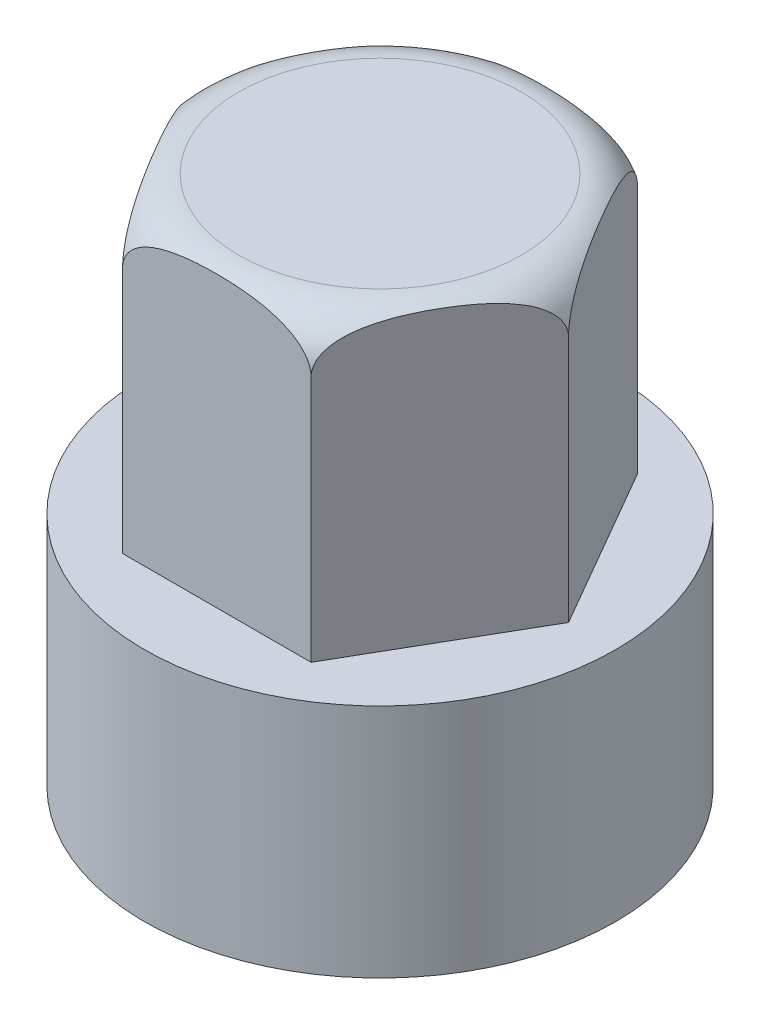
SolidWorks part; units mm, degrees
material "Plain Carbon Steel"
ref_plane "Front Plane" through (0, 0, 0) normal (0, 0, 1) x (1, 0, 0)
ref_plane "Top Plane" through (0, 0, 0) normal (0, 1, 0) x (1, 0, 0)
ref_plane "Right Plane" through (0, 0, 0) normal (1, 0, 0) x (0, 0, -1)
sketch "Cap Profile Sketch" plane through (0, 0, 0) normal (0, 0, 1) x (1, 0, 0)
  line L0 (0, 0) -> (0, 45) construction
  line L1 (0, 0) -> (20, 0)
  line L2 (20, 0) -> (20, 20)
  line L3 (20, 20) -> (16, 20)
  line L4 (16, 20) -> (16, 41)
  line L5 (12, 45) -> (0, 45)
  line L6 (0, 0) -> (0, 45)
  arc A0 (16, 41) -> (12, 45) centre (12, 41) ccw
  dimension "D5" = 4
  dimension "D1" = 40
  dimension "D2" = 32
  dimension "D3" = 20
  dimension "D4" = 45
revolve "Cap Body Revolve" add sketch "Cap Profile Sketch" angle 360 about L0
sketch "Hex 32AF Sketch" plane through (0, 45, 0) normal (0, 1, 0) x (1, 0, 0)
  line L1 (8, 13.8564) -> (-8, 13.8564)
  line L2 (-8, 13.8564) -> (-16, 0)
  line L3 (-16, 0) -> (-8, -13.8564)
  line L4 (-8, -13.8564) -> (8, -13.8564)
  line L5 (8, -13.8564) -> (16, 0)
  line L6 (16, 0) -> (8, 13.8564)
  circle A0 centre (0, 0) radius 13.8564 construction
  dimension "D1" = 32
extrude "Hex 32AF Cut" cut sketch "Hex 32AF Sketch" against normal blind 25 flip side to cut
sketch "Hex Chamfer 30deg Sketch" plane through (0, 0, 0) normal (0, 0, 1) x (1, 0, 0)
  line L0 (0, 0) -> (0, 51.1661) construction
  line L1 (0, 0) -> (12, 0)
  line L2 (-20, 0) -> (20, 0) construction
  line L3 (12, 0) -> (12, 12)
  line L4 (12, 12) -> (9, 13.7321)
  line L5 (9, 13.7321) -> (9, 39)
  line L6 (7, 41) -> (0, 41)
  line L7 (0, 0) -> (0, 41)
  arc A0 (9, 39) -> (7, 41) centre (7, 39) ccw
  dimension "D6" = 2
  dimension "D1" = 24
  dimension "D2" = 30
  dimension "D3" = 18
  dimension "D4" = 41
  dimension "D5" = 12
revolve "Hex Top Chamfer 30deg" cut sketch "Hex Chamfer 30deg Sketch" angle 360 about L0
